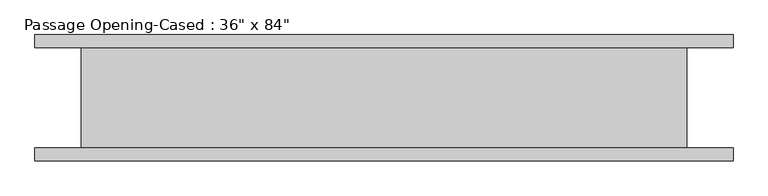
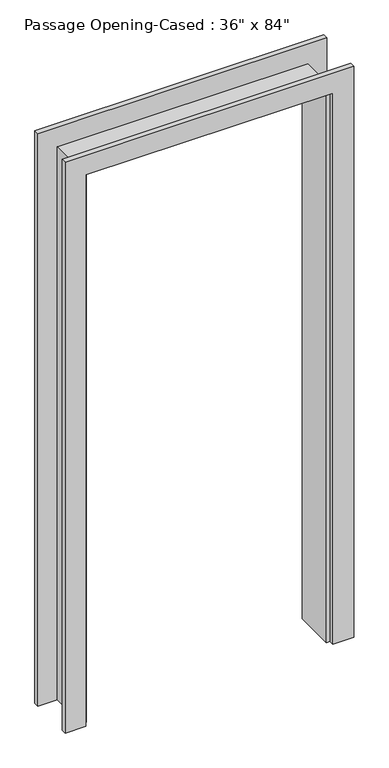
"""IFC4 building model written with IfcOpenShell, lengths in millimetres: proxy geometry."""

from ifc_helpers import new_model, si_unit, frame, origin, place, context, project, spatial, polyline, outline, extrude, faceted_brep, source, transform, mapped, element, save


def proxy_7dd6dadb(model_context):
    return source(origin(), model_context, "Body", "SolidModel", [
        faceted_brep([(429.9613433, 76.2, 0.0), (449.0113433, 76.2, 0.0), (449.0113433, -76.2, 0.0), (429.9613433, -76.2, 0.0), (429.9613433, 76.2, 2114.55), (449.0113433, 76.2, 2133.6), (449.0113433, -76.2, 2133.6), (429.9613433, -76.2, 2114.55), (-446.3386567, 76.2, 2114.55), (-465.3886567, 76.2, 2133.6), (-465.3886567, -76.2, 2133.6), (-446.3386567, -76.2, 2114.55), (-446.3386567, 76.2, 0.0), (-446.3386567, -76.2, 0.0), (-465.3886567, -76.2, 0.0), (-465.3886567, 76.2, 0.0)], [[[0, 1, 2, 3]], [[1, 0, 4, 5]], [[2, 1, 5, 6]], [[3, 2, 6, 7]], [[0, 3, 7, 4]], [[5, 4, 8, 9]], [[6, 5, 9, 10]], [[7, 6, 10, 11]], [[4, 7, 11, 8]], [[12, 13, 14, 15]], [[9, 8, 12, 15]], [[10, 9, 15, 14]], [[11, 10, 14, 13]], [[8, 11, 13, 12]]]),
        extrude(outline(polyline([(0.0, 518.8613433), (2209.8, 518.8613433), (2209.8, -535.2386567), (0.0, -535.2386567), (0.0, -459.0386567), (2127.25, -459.0386567), (2127.25, 442.6613433), (0.0, 442.6613433), (0.0, 518.8613433)])), frame((0.0, 76.2, 0.0), z_axis=(0.0, 1.0, 0.0), x_axis=(0.0, 0.0, 1.0)), (0.0, 0.0, 1.0), 19.05),
        extrude(outline(polyline([(0.0, -459.0386567), (2127.25, -459.0386567), (2127.25, 442.6613433), (0.0, 442.6613433), (0.0, 518.8613433), (2203.45, 518.8613433), (2203.45, -535.2386567), (0.0, -535.2386567), (0.0, -459.0386567)])), frame((0.0, -95.25, 0.0), z_axis=(0.0, 1.0, 0.0), x_axis=(0.0, 0.0, 1.0)), (0.0, 0.0, 1.0), 19.05),
    ])


if __name__ == "__main__":
    model = new_model("IFC4")
    model_context = context("Model", 3, world=origin())
    ifc_project = project(units=[si_unit("LENGTHUNIT", "METRE", prefix="MILLI")], contexts=[model_context])
    site = spatial("IfcSite", under=ifc_project)
    building = spatial("IfcBuilding", under=site)
    placement = place(None, origin())
    proxy_shape = proxy_7dd6dadb(model_context)
    element("IfcBuildingElementProxy", 1, Name="Passage Opening-Cased : 36\" x 84\"", ObjectType="Passage Opening-Cased : 36\" x 84\"", at=placement, inside=building, context=model_context, shape_type="MappedRepresentation", body=[
        mapped(proxy_shape, transform((0.0, 0.0, 0.0), x_axis=(1.0, 0.0, 0.0), y_axis=(0.0, 1.0, 0.0), z_axis=(0.0, 0.0, 1.0))),
    ])
    save(model, "model.ifc")

# Revit data of these elements
# Type "Passage Opening-Cased : 36\" x 84\""
#   Height = 7' - 0"
#   Trim Thickness = 0' - 0 3/4"
#   Trim Width = 0' - 3"
#   Width = 3' - 0"
#   Frame Material = Door - Frame
#   Default Elevation = 0
# Element 1 (IfcBuildingElementProxy, "Passage Opening-Cased : 36\" x 84\"")
#   Materials on its faces: "Door - Frame"
# Materials
#   "Door - Frame": colour RGB 118 70 51, transparency 0, Cost = 0
